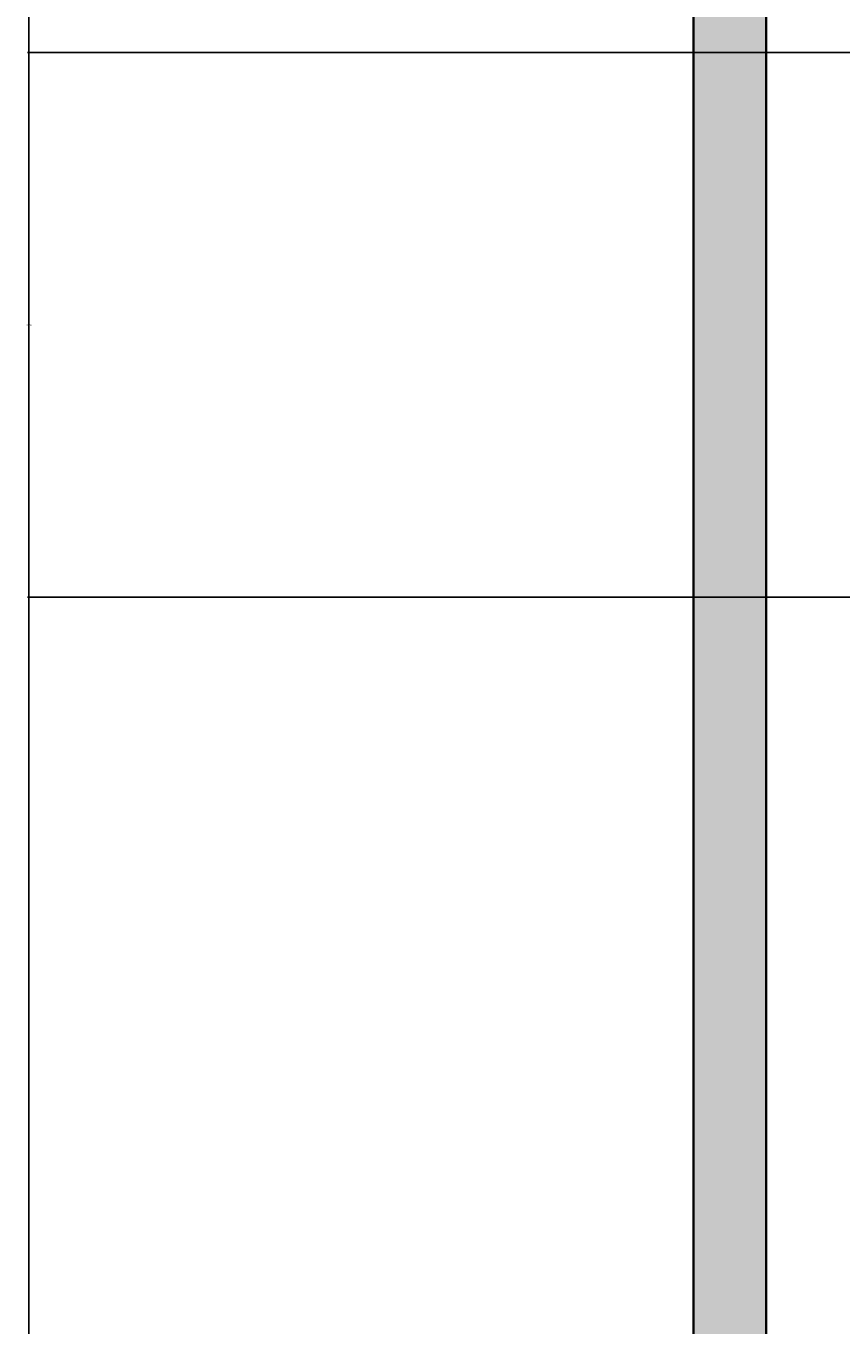
# Model space of a CAD drawing. Units: inches. Extents: x 192 to 1361, y -1362 to 367.
# Tile 6 of 23: x 192 to 293, y -616 to -454. Entities that reach past the tile are written whole.
import ezdxf

# ---------------------------------------------------------------- set-up
doc = ezdxf.new("R2010")
doc.units = ezdxf.units.IN
doc.header["$MEASUREMENT"] = 0
for name, color, linetype, lineweight in [('A-ANNO-DIMS', 2, 'Continuous', 18), ('A-WALL-PATT', 250, 'Continuous', 13), ('walls', 7, 'Continuous', 35)]:
    doc.layers.add(name, color=color, linetype=linetype, lineweight=lineweight)
doc.styles.get("Standard").update_dxf_attribs({"font": 'arial.ttf'})
doc.dimstyles.get("Standard").update_dxf_attribs({"dimtxt": 0.18, "dimasz": 0.18, "dimexe": 0.18, "dimexo": 0.0625, "dimgap": 0.09, "dimtad": 0, "dimtih": 1, "dimtoh": 1, "dimzin": 0, "dimdsep": 46, "dimlunit": 3, "dimtxsty": 'Standard', "dimcen": 0.09, "dimadec": 0, "dimazin": 0, "dimtfac": 1, "dimtofl": 0, "dimtmove": 0, "dimatfit": 3, "dimfxl": 1, "dimtolj": 1, "dimtzin": 0, "dimarcsym": 0})

# ---------------------------------------------------------------- blocks, each defined once
blk = doc.blocks.new('*D48')
at = {"layer": 'A-ANNO-DIMS', "color": 0, "lineweight": -2, "transparency": 16777216}
for p, q in [((325.63, 258.53), (192.16, 258.53)), ((192.34, 258.35), (192.34, -429.22)), ((192.34, -1117.14), (192.34, -429.58)), ((395.21, -1117.32), (192.16, -1117.32))]:
    blk.add_line(p, q, dxfattribs=at)
at = {"layer": 'A-ANNO-DIMS', "color": 0, "transparency": 16777216}
for points in [[(192.31, 258.35), (192.37, 258.35), (192.34, 258.53)], [(192.31, -1117.14), (192.37, -1117.14), (192.34, -1117.32)]]:
    blk.add_solid(points, dxfattribs=at)
at = {"layer": 'Defpoints', "color": 0, "transparency": 16777216}
for p in [(325.7, 258.53), (192.34, -1117.32), (395.28, -1117.32)]:
    blk.add_point(p, dxfattribs=at)
at = {"layer": 'A-ANNO-DIMS', "color": 0, "transparency": 16777216, "insert": (192.34, -429.4), "char_height": 0.18, "attachment_point": 5}
blk.add_mtext('\\A1;1375.9', dxfattribs=at)
blk = doc.blocks.new('*D69')
at = {"layer": 'A-ANNO-DIMS', "color": 0, "lineweight": -2, "transparency": 16777216}
for p, q in [((981.75, -457.5), (192.16, -457.5)), ((192.34, -457.68), (192.34, -491.13)), ((192.34, -524.95), (192.34, -491.5)), ((980.52, -525.13), (192.16, -525.13))]:
    blk.add_line(p, q, dxfattribs=at)
at = {"layer": 'A-ANNO-DIMS', "color": 0, "transparency": 16777216}
for points in [[(192.31, -457.68), (192.37, -457.68), (192.34, -457.5)], [(192.31, -524.95), (192.37, -524.95), (192.34, -525.13)]]:
    blk.add_solid(points, dxfattribs=at)
at = {"layer": 'Defpoints', "color": 0, "transparency": 16777216}
for p in [(981.81, -457.5), (192.34, -525.13), (980.58, -525.13)]:
    blk.add_point(p, dxfattribs=at)
at = {"layer": 'A-ANNO-DIMS', "color": 0, "transparency": 16777216, "insert": (192.34, -491.31), "char_height": 0.18, "attachment_point": 5}
blk.add_mtext('\\A1;67.63', dxfattribs=at)

msp = doc.modelspace()

# ---------------------------------------------------------------- hatches: boundary and pattern name
at = {"layer": 'A-WALL-PATT'}
h = msp.add_hatch(color=256, dxfattribs=at)
h.dxf.hatch_style = 1
h.paths.add_polyline_path([(309.5452, 191.102), (300.5452, 191.102), (300.5452, -126.898), (309.5452, -126.898), (309.5452, -117.898)])
h.paths.add_polyline_path([(420.798, 191.102), (337.3229, 191.102), (337.3229, 182.102), (420.798, 182.102)])
h.paths.add_polyline_path([(518.5452, 182.102), (625.4022, 182.102), (625.4022, 191.102), (509.5452, 191.102), (509.5452, 114.3262), (518.5452, 114.3262)])
h.paths.add_polyline_path([(842.5452, 191.102), (763.4438, 191.102), (763.4438, 182.102), (833.5452, 182.102), (833.5452, 161.1615), (836.8088, 161.1615), (842.5452, 161.1615)])
h.paths.add_polyline_path([(842.5452, -16.5675), (833.5452, -16.5675), (833.5452, -60.4996), (784.8041, -60.4996), (784.8041, -354.6796), (793.8041, -354.6796), (793.8041, -69.4996), (1094.1252, -69.4996), (1094.1252, -60.4996), (842.5452, -60.4996)])
h.paths.add_polyline_path([(518.5452, 36.602), (509.5452, 36.602), (509.5452, -117.898), (420.2204, -117.898), (420.2204, -126.898), (518.5452, -126.898)])
h.paths.add_polyline_path([(474.8041, -377.0384), (465.8041, -377.0384), (465.8041, -381.5384), (465.8041, -450.898), (537.5717, -450.898), (537.5717, -441.898), (474.8041, -441.898)])
h.paths.add_polyline_path([(1162.8041, -380.6763), (1204.3001, -380.6763), (1204.3001, -375.6763), (1195.1471, -375.6763), (1153.8041, -375.6763), (1153.8041, -448.4996), (856.5691, -448.4996), (856.5691, -457.4996), (1162.8041, -457.4996)])
h.paths.add_polyline_path([(1162.8041, -525.128), (1153.8041, -525.128), (1153.8041, -597.4996), (1162.8041, -597.4996)], flags=17)
h.paths.add_polyline_path([(1162.8041, -60.4996), (1153.8041, -60.4996), (1153.8041, -69.4996), (1153.8041, -177.4733), (1205.8889, -177.4733), (1205.8889, -172.4733), (1162.8041, -172.4733)])
h.paths.add_polyline_path([(980.5799, -525.686), (971.5799, -525.686), (971.5799, -597.4996), (980.5799, -597.4996)], flags=17)
h.paths.add_polyline_path([(856.5691, -448.4996), (798.7542, -448.4996), (784.8041, -448.4996), (784.8041, -457.4996), (847.5691, -457.4996), (847.5691, -597.4996), (784.8041, -597.4996), (784.8041, -606.4996), (1273.5658, -606.4996), (1273.5658, -597.4996), (856.5691, -597.4996)])
h.paths.add_polyline_path([(1273.5658, -773.892), (1099.8366, -773.892), (1099.8366, -851.9362), (1108.8366, -851.9362), (1108.8366, -782.892), (1273.5658, -782.892)])
h.paths.add_polyline_path([(1108.8366, -982.9214), (1099.8366, -982.9214), (1099.8366, -1067.6246), (1037.7563, -1067.6246), (1037.7563, -1076.6246), (1108.8366, -1076.6246)])
h.paths.add_polyline_path([(835.078, -1067.6246), (758.8458, -1067.6246), (758.8458, -940.2324), (749.8458, -940.2324), (749.8458, -963.172), (749.8458, -970.4644), (749.8458, -1076.6246), (835.078, -1076.6246)])
h.paths.add_polyline_path([(450.307, -1066.9838), (441.307, -1066.9838), (441.307, -1076.6246), (450.307, -1076.6246)])
h.paths.add_polyline_path([(492.8925, -756.4415), (274.8925, -756.4415), (274.8925, -765.4415), (492.8925, -765.4415)])
h.paths.add_polyline_path([(283.8925, -835.2244), (274.8925, -835.2244), (274.8925, -914.4415), (492.8925, -914.4415), (492.8925, -839.9415), (483.8925, -839.9415), (483.8925, -905.4415), (283.8925, -905.4415)])
h.paths.add_polyline_path([(283.8925, -441.898), (283.8925, -375.4296), (281.6021, -375.4296), (281.6021, -399.4121), (274.8925, -399.4121), (274.8925, -441.898), (274.8925, -684.5089), (283.8925, -684.5089)])

# ---------------------------------------------------------------- linework, layer by layer
at = {"layer": 'walls'}
for p, q in [((274.8925, -441.898), (274.8925, -914.4415)), ((283.8925, -441.898), (283.8925, -756.4415))]:
    msp.add_line(p, q, dxfattribs=at)

# ---------------------------------------------------------------- dimensions: what is measured, and where the dimension line sits
at = {"layer": 'A-ANNO-DIMS'}
for base, p1, p2, override, picture, middle in [((192.3425, -1117.3227), (325.6957, 258.5286), (395.2768, -1117.3227), {"dimdec": 1, "dimlfac": 1, "dimrnd": 0, "dimzin": 0, "dimdsep": 46, "dimlunit": 2}, '*D48', (192.3425, -429.3971)), ((192.3425, -525.128), (981.8078, -457.4996), (980.5799, -525.128), {"dimdec": 2, "dimlfac": 1, "dimrnd": 0, "dimzin": 0, "dimdsep": 46, "dimlunit": 2}, '*D69', (192.3425, -491.3138))]:
    dim = msp.add_linear_dim(base=base, p1=p1, p2=p2, angle=90, dimstyle='Standard', override=override, dxfattribs=at)
    dim.commit()
    dim.dimension.update_dxf_attribs({"geometry": picture, "text_midpoint": middle})

doc.saveas('drawing.dxf')
